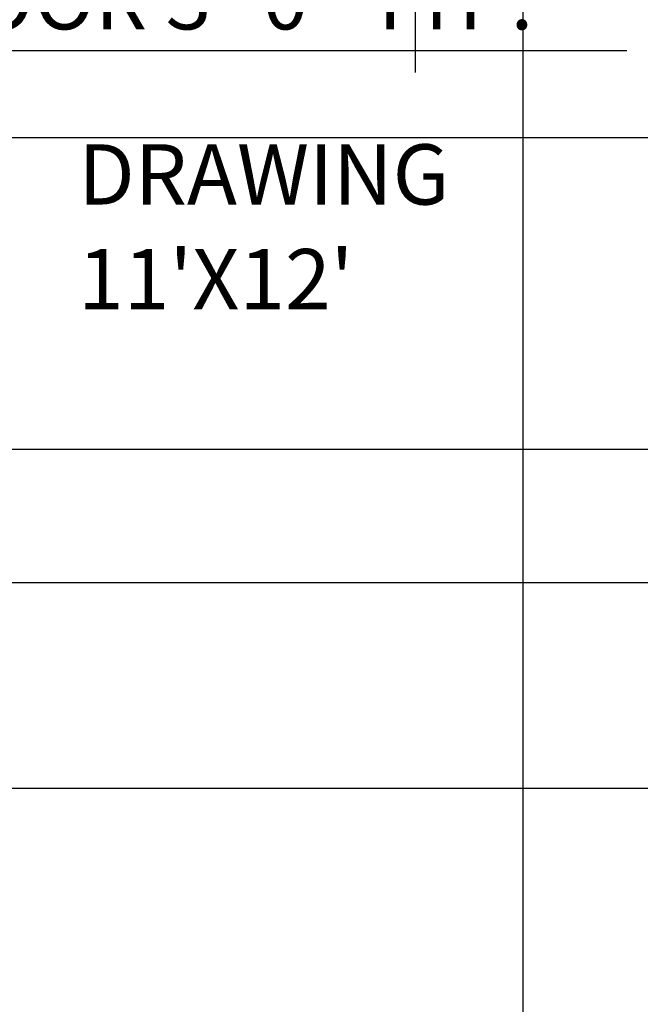
# Model space of a CAD drawing. Units: inches. Extents: x 2923 to 3500, y 1684 to 2381.
# Tile 3 of 12: x 3125 to 3176, y 1848 to 1930. Entities that reach past the tile are written whole.
import ezdxf

# ---------------------------------------------------------------- set-up
doc = ezdxf.new("R2010")
doc.units = ezdxf.units.IN
doc.layers.add('A-ANNO-DIMS', color=2, linetype='Continuous', lineweight=18)
doc.layers.add('A-AREA-IDEN', color=7, linetype='Continuous', lineweight=18)
doc.styles.get("Standard").update_dxf_attribs({"font": 'txt', "height": 5})
doc.dimstyles.new('ISO-25', dxfattribs={"dimtxt": 5, "dimasz": 2.5, "dimexe": 1.25, "dimexo": 0.625, "dimtad": 1, "dimlunit": 3, "dimtxsty": 'Standard', "dimcen": 2.5, "dimadec": 0, "dimazin": 0, "dimtfac": 1, "dimtmove": 0, "dimatfit": 3, "dimfxl": 1, "dimarcsym": 0})

# ---------------------------------------------------------------- blocks, each defined once
blk = doc.blocks.new('*D25')
at = {"layer": 'A-ANNO-DIMS', "color": 0, "lineweight": -2, "transparency": 16777216}
for p, q in [((3069.73, 1931.781), (3069.73, 1925.756)), ((3105.73, 1931.781), (3105.73, 1925.756)), ((3072.23, 1927.006), (3103.23, 1927.006)), ((3105.73, 1927.006), (3174.956, 1927.006))]:
    blk.add_line(p, q, dxfattribs=at)
at = {"layer": 'A-ANNO-DIMS', "color": 0, "transparency": 16777216}
for points in [[(3072.23, 1927.423), (3072.23, 1926.59), (3069.73, 1927.006)], [(3103.23, 1927.423), (3103.23, 1926.59), (3105.73, 1927.006)]]:
    blk.add_solid(points, dxfattribs=at)
at = {"layer": 'Defpoints', "color": 0, "transparency": 16777216}
for p in [(3069.73, 1932.406), (3105.73, 1932.406), (3105.73, 1927.006)]:
    blk.add_point(p, dxfattribs=at)
at = {"layer": 'A-ANNO-DIMS', "color": 0, "transparency": 16777216, "insert": (3141.593, 1930.607), "char_height": 5, "attachment_point": 5}
blk.add_mtext('DOOR 3\'-0" TYP.', dxfattribs=at)
blk = doc.blocks.new('*D39')
at = {"layer": 'A-ANNO-DIMS', "color": 0, "lineweight": -2, "transparency": 16777216}
for p, q in [((3159.845, 2034.288), (3156.13, 2034.288)), ((3157.38, 2031.788), (3157.38, 2016.183)), ((3159.845, 2013.683), (3156.13, 2013.683)), ((3157.38, 2013.683), (3157.38, 1925.171))]:
    blk.add_line(p, q, dxfattribs=at)
at = {"layer": 'A-ANNO-DIMS', "color": 0, "transparency": 16777216}
for points in [[(3156.963, 2031.788), (3157.796, 2031.788), (3157.38, 2034.288)], [(3156.963, 2016.183), (3157.796, 2016.183), (3157.38, 2013.683)]]:
    blk.add_solid(points, dxfattribs=at)
at = {"layer": 'Defpoints', "color": 0, "transparency": 16777216}
for p in [(3160.47, 2034.288), (3157.38, 2013.683), (3160.47, 2013.683)]:
    blk.add_point(p, dxfattribs=at)
at = {"layer": 'A-ANNO-DIMS', "color": 0, "transparency": 16777216, "insert": (3152.945, 1968.177), "char_height": 5, "attachment_point": 5, "rotation": 90}
blk.add_mtext('CHAIR 1\'-8 1/2" TYP.', dxfattribs=at)
blk = doc.blocks.new('*D54')
at = {"layer": 'A-ANNO-DIMS', "color": 0, "lineweight": -2, "transparency": 16777216}
for p, q in [((3166.316, 2236.755), (3166.316, 1685.656)), ((3193.644, 2236.755), (3193.644, 1685.656)), ((3168.816, 1686.906), (3191.144, 1686.906)), ((3193.644, 1686.906), (3235.489, 1686.906))]:
    blk.add_line(p, q, dxfattribs=at)
at = {"layer": 'A-ANNO-DIMS', "color": 0, "transparency": 16777216}
for points in [[(3168.816, 1687.323), (3168.816, 1686.49), (3166.316, 1686.906)], [(3191.144, 1687.323), (3191.144, 1686.49), (3193.644, 1686.906)]]:
    blk.add_solid(points, dxfattribs=at)
at = {"layer": 'Defpoints', "color": 0, "transparency": 16777216}
for p in [(3166.316, 2237.38), (3193.644, 2237.38), (3193.644, 1686.906)]:
    blk.add_point(p, dxfattribs=at)
at = {"layer": 'A-ANNO-DIMS', "color": 0, "transparency": 16777216, "insert": (3215.817, 1691.341), "char_height": 5, "attachment_point": 5}
blk.add_mtext('2\'-3 1/2"', dxfattribs=at)
blk = doc.blocks.new('*D63')
at = {"layer": 'A-ANNO-DIMS', "color": 0, "lineweight": -2, "transparency": 16777216}
for p, q in [((3203.709, 1919.766), (2933.48, 1919.766)), ((2934.73, 1896.412), (2934.73, 1917.266)), ((3203.709, 1893.912), (2933.48, 1893.912))]:
    blk.add_line(p, q, dxfattribs=at)
at = {"layer": 'A-ANNO-DIMS', "color": 0, "transparency": 16777216}
for points in [[(2934.313, 1917.266), (2935.146, 1917.266), (2934.73, 1919.766)], [(2934.313, 1896.412), (2935.146, 1896.412), (2934.73, 1893.912)]]:
    blk.add_solid(points, dxfattribs=at)
at = {"layer": 'Defpoints', "color": 0, "transparency": 16777216}
for p in [(2934.73, 1919.766), (3204.334, 1919.766), (3204.334, 1893.912)]:
    blk.add_point(p, dxfattribs=at)
at = {"layer": 'A-ANNO-DIMS', "color": 0, "transparency": 16777216, "insert": (2931.129, 1906.839), "char_height": 5, "attachment_point": 5, "rotation": 90}
blk.add_mtext('2\'-2"', dxfattribs=at)
blk = doc.blocks.new('*D65')
at = {"layer": 'A-ANNO-DIMS', "color": 0, "lineweight": -2, "transparency": 16777216}
for p, q in [((2934.73, 1882.852), (2934.73, 1905.411)), ((3193.074, 1882.852), (2933.48, 1882.852)), ((2934.73, 1868.288), (2934.73, 1880.352)), ((3193.074, 1865.788), (2933.48, 1865.788))]:
    blk.add_line(p, q, dxfattribs=at)
at = {"layer": 'A-ANNO-DIMS', "color": 0, "transparency": 16777216}
for points in [[(2934.313, 1880.352), (2935.146, 1880.352), (2934.73, 1882.852)], [(2934.313, 1868.288), (2935.146, 1868.288), (2934.73, 1865.788)]]:
    blk.add_solid(points, dxfattribs=at)
at = {"layer": 'Defpoints', "color": 0, "transparency": 16777216}
for p in [(2934.73, 1882.852), (3193.699, 1882.852), (3193.699, 1865.788)]:
    blk.add_point(p, dxfattribs=at)
at = {"layer": 'A-ANNO-DIMS', "color": 0, "transparency": 16777216, "insert": (2931.129, 1895.382), "char_height": 5, "attachment_point": 5, "rotation": 90}
blk.add_mtext('1\'-5"', dxfattribs=at)

msp = doc.modelspace()

# ---------------------------------------------------------------- texts
at = {"layer": 'A-AREA-IDEN'}
for s, p in [('DRAWING', (3129.418, 1914.229)), ("11'X12'", (3129.418, 1905.544))]:
    msp.add_text(s, height=5, dxfattribs=at).set_placement(p)

# ---------------------------------------------------------------- dimensions: what is measured, and where the dimension line sits
at = {"layer": 'A-ANNO-DIMS'}
dim = msp.add_linear_dim(base=(3193.644, 1686.906), p1=(3166.316, 2237.38), p2=(3193.644, 2237.38), dimstyle='ISO-25', override={"dimdec": 1, "dimlfac": 1, "dimrnd": 0, "dimzin": 1, "dimdsep": 46, "dimlunit": 4, "dimfrac": 2}, dxfattribs=at)
dim.commit()
dim.dimension.update_dxf_attribs({"geometry": '*D54', "text_midpoint": (3215.817, 1691.341)})
dim = msp.add_linear_dim(base=(3157.38, 2013.683), p1=(3160.47, 2034.288), p2=(3160.47, 2013.683), angle=270, text='CHAIR <> TYP.', dimstyle='ISO-25', override={"dimdec": 1, "dimlfac": 1, "dimrnd": 0, "dimzin": 1, "dimdsep": 46, "dimlunit": 4, "dimfrac": 2}, dxfattribs=at)
dim.commit()
dim.dimension.update_dxf_attribs({"geometry": '*D39', "text_midpoint": (3152.945, 1968.177)})
dim = msp.add_linear_dim(base=(3105.73, 1927.006), p1=(3069.73, 1932.406), p2=(3105.73, 1932.406), text='DOOR <> TYP.', dimstyle='ISO-25', override={"dimdec": 1, "dimlfac": 1, "dimrnd": 0, "dimzin": 1, "dimdsep": 46, "dimlunit": 4, "dimfrac": 2}, dxfattribs=at)
dim.commit()
dim.dimension.update_dxf_attribs({"geometry": '*D25', "text_midpoint": (3141.593, 1930.607)})
for base, p1, p2, picture, middle in [((2934.73, 1919.766), (3204.334, 1893.912), (3204.334, 1919.766), '*D63', (2931.129, 1906.839)), ((2934.73, 1882.852), (3193.699, 1865.788), (3193.699, 1882.852), '*D65', (2931.129, 1895.382))]:
    dim = msp.add_linear_dim(base=base, p1=p1, p2=p2, angle=90, dimstyle='ISO-25', override={"dimdec": 1, "dimlfac": 1, "dimrnd": 0, "dimzin": 1, "dimdsep": 46, "dimlunit": 4, "dimfrac": 2}, dxfattribs=at)
    dim.commit()
    dim.dimension.update_dxf_attribs({"geometry": picture, "text_midpoint": middle})

doc.saveas('drawing.dxf')
